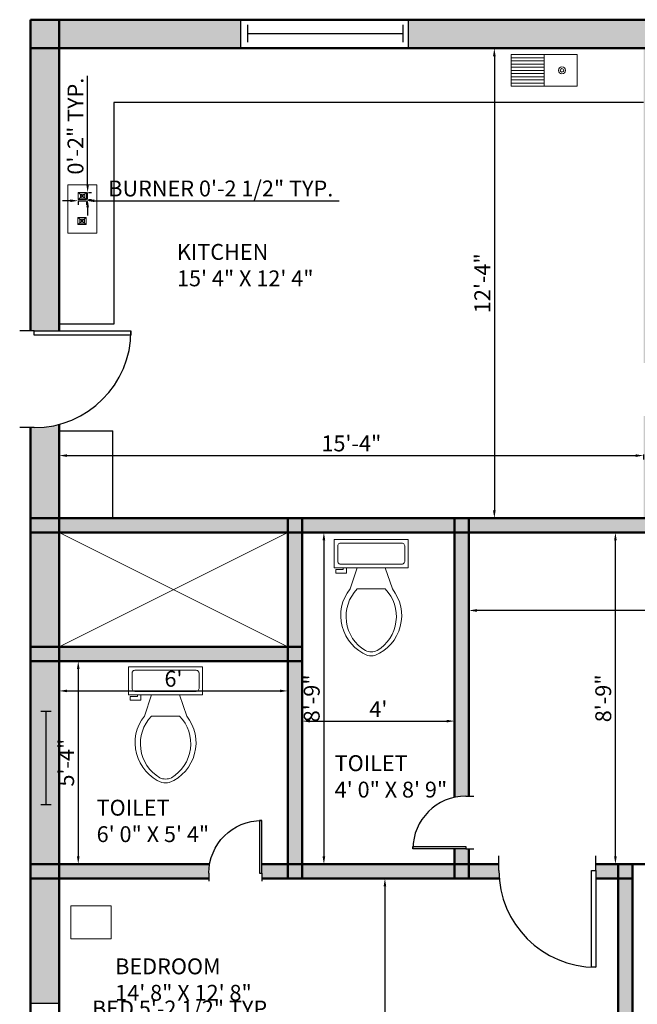
# Model space of a CAD drawing. Units: millimetres. Extents: x 3107 to 3757, y 777 to 1464.
# Tile 4 of 7: x 3107 to 3301, y 1140 to 1450. Entities that reach past the tile are written whole.
import ezdxf

# ---------------------------------------------------------------- set-up
doc = ezdxf.new("R2010")
doc.units = ezdxf.units.MM
for name, color, linetype, lineweight in [('A-ANNO-DIMS', 50, 'Continuous', 18), ('A-AREA-IDEN', 160, 'Continuous', 18), ('A-EQPM', 140, 'Continuous', 18), ('A-FLOR-CASE', 140, 'Continuous', 25), ('A-FLOR-FIXT', 140, 'Continuous', 18), ('A-FLOR-OPEN', 8, 'Continuous', 18), ('A-WALL-PATT', 80, 'Continuous', 13), ('doors', 10, 'Continuous', 25), ('furniture', 140, 'Continuous', 18), ('walls', 80, 'Continuous', 50), ('windows', 30, 'Continuous', 25)]:
    doc.layers.add(name, color=color, linetype=linetype, lineweight=lineweight)
doc.styles.get("Standard").update_dxf_attribs({"font": 'arial.ttf'})
doc.dimstyles.new('ISO-25', dxfattribs={"dimtxt": 5, "dimasz": 2.5, "dimexe": 1.25, "dimexo": 0.625, "dimtad": 1, "dimdec": 0, "dimlunit": 3, "dimtxsty": 'Standard', "dimcen": 2.5, "dimadec": 0, "dimazin": 0, "dimtfac": 1, "dimtdec": 0, "dimtmove": 0, "dimatfit": 3, "dimfxl": 1, "dimarcsym": 0})

# ---------------------------------------------------------------- blocks, each defined once
blk = doc.blocks.new('*U2')
for p, q in [((0, 0), (0, -6)), ((40, 0), (40, -6))]:
    blk.add_line(p, q)
blk.add_lwpolyline([(0, 0), (0, 40), (1.75, 40), (1.75, 0)], close=True)
blk.add_arc((0, 0), 40, 0, 90)
blk = doc.blocks.new('*U4')
for p, q in [((0, 4), (0, 0)), ((36, 4), (36, 0)), ((0, 2), (36, 2))]:
    blk.add_line(p, q)
blk = doc.blocks.new('*U5')
for p, q in [((0, 4), (0, 0)), ((36, 4), (36, 0)), ((0, 2), (36, 2))]:
    blk.add_line(p, q)
blk = doc.blocks.new('Toilet - top')
for p, q in [((9.5, -6), (9.5, -2)), ((-8, -8.5), (-8, -8)), ((-7, -8), (-7, -9.5)), ((-4, -8), (-6, -14)), ((4, -8), (6, -14)), ((-10, -8.5), (-8, -8.5)), ((-10, -9.5), (-10, -8.5)), ((-7, -9.5), (-10, -9.5)), ((4, -14), (-4, -14))]:
    blk.add_line(p, q)
blk.add_lwpolyline([(10.5, -8), (10.5, 0), (-10.5, 0), (-10.5, -8)], close=True)
for points in [[(-9.5, -2), (-9.5, -6)], [(8.5, -1), (-8.5, -1)], [(-8.5, -7), (8.5, -7)]]:
    blk.add_lwpolyline(points)
for centre, radius, start, end in [((-8.62, -1.88), 0.884, 81.8699, 188.1301), ((8.62, -1.88), 0.884, 351.8699, 98.1301), ((-8.62, -6.12), 0.884, 171.8699, 278.1301), ((8.62, -6.12), 0.884, 261.8699, 8.1301), ((3.52, -21.58), 12.17, 141.4691, 247.9714), ((4.2, -21.82), 11.33, 136.3677, 238.9468), ((-3.52, -21.58), 12.17, 292.0284, 38.5307), ((-4.2, -21.82), 11.33, 301.053, 43.6321), ((0, -27.88), 4, 245.7318, 294.2682), ((0, -29), 4, 254.8605, 285.1395)]:
    blk.add_arc(centre, radius, start, end)
blk = doc.blocks.new('*D16')
at = {"layer": 'A-ANNO-DIMS', "color": 0, "lineweight": -2, "transparency": 16777216}
for p, q in [((3257.1, 1441.43), (3257.73, 1441.43)), ((3256.48, 1438.93), (3256.48, 1295.93)), ((3257.1, 1293.43), (3257.73, 1293.43))]:
    blk.add_line(p, q, dxfattribs=at)
at = {"layer": 'A-ANNO-DIMS', "color": 0, "transparency": 16777216}
for points in [[(3256.06, 1438.93), (3256.9, 1438.93), (3256.48, 1441.43)], [(3256.06, 1295.93), (3256.9, 1295.93), (3256.48, 1293.43)]]:
    blk.add_solid(points, dxfattribs=at)
at = {"layer": 'Defpoints', "color": 0, "transparency": 16777216}
for p in [(3256.48, 1441.43), (3256.48, 1293.43), (3256.48, 1293.43)]:
    blk.add_point(p, dxfattribs=at)
at = {"layer": 'A-ANNO-DIMS', "color": 0, "transparency": 16777216, "insert": (3253.34, 1367.43), "char_height": 5, "attachment_point": 5, "rotation": 90}
blk.add_mtext('12\'-4"', dxfattribs=at)
blk = doc.blocks.new('*D17')
at = {"layer": 'A-ANNO-DIMS', "color": 0, "lineweight": -2, "transparency": 16777216}
for p, q in [((3119.47, 1311.37), (3119.47, 1314.39)), ((3121.97, 1313.14), (3300.97, 1313.14)), ((3303.47, 1313.51), (3303.47, 1311.89))]:
    blk.add_line(p, q, dxfattribs=at)
at = {"layer": 'A-ANNO-DIMS', "color": 0, "transparency": 16777216}
for points in [[(3121.97, 1313.56), (3121.97, 1312.72), (3119.47, 1313.14)], [(3300.97, 1313.56), (3300.97, 1312.72), (3303.47, 1313.14)]]:
    blk.add_solid(points, dxfattribs=at)
at = {"layer": 'Defpoints', "color": 0, "transparency": 16777216}
for p in [(3303.47, 1314.14), (3303.47, 1313.14), (3119.47, 1310.75)]:
    blk.add_point(p, dxfattribs=at)
at = {"layer": 'A-ANNO-DIMS', "color": 0, "transparency": 16777216, "insert": (3211.47, 1316.32), "char_height": 5, "attachment_point": 5}
blk.add_mtext('15\'-4"', dxfattribs=at)
blk = doc.blocks.new('*D24')
at = {"layer": 'A-ANNO-DIMS', "color": 0, "lineweight": -2, "transparency": 16777216}
for p, q in [((3248.47, 1264.98), (3248.47, 1265.6)), ((3464.47, 1264.98), (3464.47, 1265.6)), ((3461.97, 1264.35), (3250.97, 1264.35))]:
    blk.add_line(p, q, dxfattribs=at)
at = {"layer": 'A-ANNO-DIMS', "color": 0, "transparency": 16777216}
for points in [[(3250.97, 1264.77), (3250.97, 1263.94), (3248.47, 1264.35)], [(3461.97, 1264.77), (3461.97, 1263.94), (3464.47, 1264.35)]]:
    blk.add_solid(points, dxfattribs=at)
at = {"layer": 'Defpoints', "color": 0, "transparency": 16777216}
for p in [(3248.47, 1264.35), (3248.47, 1264.35), (3464.47, 1264.35)]:
    blk.add_point(p, dxfattribs=at)
at = {"layer": 'A-ANNO-DIMS', "color": 0, "transparency": 16777216, "insert": (3356.47, 1267.53), "char_height": 5, "attachment_point": 5}
blk.add_mtext("18'", dxfattribs=at)
blk = doc.blocks.new('*D25')
at = {"layer": 'A-ANNO-DIMS', "color": 0, "lineweight": -2, "transparency": 16777216}
for p, q in [((3294.84, 1288.93), (3293.35, 1288.93)), ((3294.6, 1186.93), (3294.6, 1286.43)), ((3294.84, 1184.43), (3293.35, 1184.43))]:
    blk.add_line(p, q, dxfattribs=at)
at = {"layer": 'A-ANNO-DIMS', "color": 0, "transparency": 16777216}
for points in [[(3294.18, 1286.43), (3295.01, 1286.43), (3294.6, 1288.93)], [(3294.18, 1186.93), (3295.01, 1186.93), (3294.6, 1184.43)]]:
    blk.add_solid(points, dxfattribs=at)
at = {"layer": 'Defpoints', "color": 0, "transparency": 16777216}
for p in [(3294.6, 1288.93), (3295.47, 1288.93), (3295.47, 1184.43)]:
    blk.add_point(p, dxfattribs=at)
at = {"layer": 'A-ANNO-DIMS', "color": 0, "transparency": 16777216, "insert": (3291.42, 1236.68), "char_height": 5, "attachment_point": 5, "rotation": 90}
blk.add_mtext('8\'-9"', dxfattribs=at)
blk = doc.blocks.new('*D26')
at = {"layer": 'A-ANNO-DIMS', "color": 0, "lineweight": -2, "transparency": 16777216}
for p, q in [((3195.97, 1225.71), (3195.97, 1230.76)), ((3198.47, 1229.51), (3241.47, 1229.51)), ((3243.97, 1225.71), (3243.97, 1230.76))]:
    blk.add_line(p, q, dxfattribs=at)
at = {"layer": 'A-ANNO-DIMS', "color": 0, "transparency": 16777216}
for points in [[(3198.47, 1229.92), (3198.47, 1229.09), (3195.97, 1229.51)], [(3241.47, 1229.92), (3241.47, 1229.09), (3243.97, 1229.51)]]:
    blk.add_solid(points, dxfattribs=at)
at = {"layer": 'Defpoints', "color": 0, "transparency": 16777216}
for p in [(3243.97, 1229.51), (3195.97, 1225.08), (3243.97, 1225.08)]:
    blk.add_point(p, dxfattribs=at)
at = {"layer": 'A-ANNO-DIMS', "color": 0, "transparency": 16777216, "insert": (3219.97, 1232.63), "char_height": 5, "attachment_point": 5}
blk.add_mtext("4'", dxfattribs=at)
blk = doc.blocks.new('*D27')
at = {"layer": 'A-ANNO-DIMS', "color": 0, "lineweight": -2, "transparency": 16777216}
for p, q in [((3200.33, 1288.93), (3204.07, 1288.93)), ((3202.82, 1286.43), (3202.82, 1186.93)), ((3200.33, 1184.43), (3204.07, 1184.43))]:
    blk.add_line(p, q, dxfattribs=at)
at = {"layer": 'A-ANNO-DIMS', "color": 0, "transparency": 16777216}
for points in [[(3202.4, 1286.43), (3203.24, 1286.43), (3202.82, 1288.93)], [(3202.4, 1186.93), (3203.24, 1186.93), (3202.82, 1184.43)]]:
    blk.add_solid(points, dxfattribs=at)
at = {"layer": 'Defpoints', "color": 0, "transparency": 16777216}
for p in [(3199.7, 1288.93), (3199.7, 1184.43), (3202.82, 1184.43)]:
    blk.add_point(p, dxfattribs=at)
at = {"layer": 'A-ANNO-DIMS', "color": 0, "transparency": 16777216, "insert": (3199.64, 1236.68), "char_height": 5, "attachment_point": 5, "rotation": 90}
blk.add_mtext('8\'-9"', dxfattribs=at)
blk = doc.blocks.new('*D28')
at = {"layer": 'A-ANNO-DIMS', "color": 0, "lineweight": -2, "transparency": 16777216}
for p, q in [((3119.47, 1241.1), (3119.47, 1237.77)), ((3191.47, 1241.1), (3191.47, 1237.77)), ((3121.97, 1239.02), (3188.97, 1239.02))]:
    blk.add_line(p, q, dxfattribs=at)
at = {"layer": 'A-ANNO-DIMS', "color": 0, "transparency": 16777216}
for points in [[(3121.97, 1239.44), (3121.97, 1238.61), (3119.47, 1239.02)], [(3188.97, 1239.44), (3188.97, 1238.61), (3191.47, 1239.02)]]:
    blk.add_solid(points, dxfattribs=at)
at = {"layer": 'Defpoints', "color": 0, "transparency": 16777216}
for p in [(3119.47, 1241.72), (3191.47, 1241.72), (3191.47, 1239.02)]:
    blk.add_point(p, dxfattribs=at)
at = {"layer": 'A-ANNO-DIMS', "color": 0, "transparency": 16777216, "insert": (3155.47, 1242.2), "char_height": 5, "attachment_point": 5}
blk.add_mtext("6'", dxfattribs=at)
blk = doc.blocks.new('*D29')
at = {"layer": 'A-ANNO-DIMS', "color": 0, "lineweight": -2, "transparency": 16777216}
for p, q in [((3123.55, 1248.43), (3126.75, 1248.43)), ((3125.5, 1245.93), (3125.5, 1186.93)), ((3123.55, 1184.43), (3126.75, 1184.43))]:
    blk.add_line(p, q, dxfattribs=at)
at = {"layer": 'A-ANNO-DIMS', "color": 0, "transparency": 16777216}
for points in [[(3125.08, 1245.93), (3125.91, 1245.93), (3125.5, 1248.43)], [(3125.08, 1186.93), (3125.91, 1186.93), (3125.5, 1184.43)]]:
    blk.add_solid(points, dxfattribs=at)
at = {"layer": 'Defpoints', "color": 0, "transparency": 16777216}
for p in [(3122.92, 1248.43), (3122.92, 1184.43), (3125.5, 1184.43)]:
    blk.add_point(p, dxfattribs=at)
at = {"layer": 'A-ANNO-DIMS', "color": 0, "transparency": 16777216, "insert": (3122.33, 1216.43), "char_height": 5, "attachment_point": 5, "rotation": 90}
blk.add_mtext('5\'-4"', dxfattribs=at)
blk = doc.blocks.new('*D33')
at = {"layer": 'A-ANNO-DIMS', "color": 0, "lineweight": -2, "transparency": 16777216}
for p, q in [((3221.28, 1179.93), (3223.29, 1179.93)), ((3222.04, 1177.43), (3222.04, 1030.43)), ((3221.28, 1027.93), (3223.29, 1027.93))]:
    blk.add_line(p, q, dxfattribs=at)
at = {"layer": 'A-ANNO-DIMS', "color": 0, "transparency": 16777216}
for points in [[(3221.62, 1177.43), (3222.45, 1177.43), (3222.04, 1179.93)], [(3221.62, 1030.43), (3222.45, 1030.43), (3222.04, 1027.93)]]:
    blk.add_solid(points, dxfattribs=at)
at = {"layer": 'Defpoints', "color": 0, "transparency": 16777216}
for p in [(3220.65, 1179.93), (3220.65, 1027.93), (3222.04, 1027.93)]:
    blk.add_point(p, dxfattribs=at)
at = {"layer": 'A-ANNO-DIMS', "color": 0, "transparency": 16777216, "insert": (3218.86, 1103.93), "char_height": 5, "attachment_point": 5, "rotation": 90}
blk.add_mtext('12\'-8"', dxfattribs=at)
blk = doc.blocks.new('COOKTOP-BURNER')
for p, q in [((0, 2.24), (2.56, 0)), ((2.56, 2.24), (0, 0))]:
    blk.add_line(p, q)
for points in [[(0, 2.24), (2.56, 2.24), (2.56, 0), (0, 0)], [(0.66, 1.7), (2.06, 1.7), (2.06, 0.46), (0.66, 0.46)]]:
    blk.add_lwpolyline(points, close=True)
blk = doc.blocks.new('*D49')
at = {"layer": 'A-ANNO-DIMS', "color": 0, "lineweight": -2, "transparency": 16777216}
for p, q in [((3127.01, 1126.35), (3127.01, 1136.38)), ((3187.19, 1135.13), (3129.51, 1135.13)), ((3189.69, 1126.35), (3189.69, 1136.38))]:
    blk.add_line(p, q, dxfattribs=at)
at = {"layer": 'A-ANNO-DIMS', "color": 0, "transparency": 16777216}
for points in [[(3129.51, 1135.55), (3129.51, 1134.71), (3127.01, 1135.13)], [(3187.19, 1135.55), (3187.19, 1134.71), (3189.69, 1135.13)]]:
    blk.add_solid(points, dxfattribs=at)
at = {"layer": 'Defpoints', "color": 0, "transparency": 16777216}
for p in [(3127.01, 1135.13), (3127.01, 1125.73), (3189.69, 1125.73)]:
    blk.add_point(p, dxfattribs=at)
at = {"layer": 'A-ANNO-DIMS', "color": 0, "transparency": 16777216, "insert": (3158.35, 1138.34), "char_height": 5, "attachment_point": 5}
blk.add_mtext('BED 5\'-2 1/2" TYP.', dxfattribs=at)
blk = doc.blocks.new('*D61')
at = {"layer": 'A-ANNO-DIMS', "color": 0, "lineweight": -2, "transparency": 16777216}
for p, q in [((3123, 1393.41), (3120.5, 1393.41)), ((3125.5, 1393.41), (3128.06, 1393.41)), ((3125.5, 1393.17), (3125.5, 1392.16)), ((3128.06, 1393.17), (3128.06, 1392.16)), ((3130.56, 1393.41), (3207.66, 1393.41))]:
    blk.add_line(p, q, dxfattribs=at)
at = {"layer": 'A-ANNO-DIMS', "color": 0, "transparency": 16777216}
for points in [[(3123, 1393.83), (3123, 1393), (3125.5, 1393.41)], [(3130.56, 1393.83), (3130.56, 1393), (3128.06, 1393.41)]]:
    blk.add_solid(points, dxfattribs=at)
at = {"layer": 'Defpoints', "color": 0, "transparency": 16777216}
for p in [(3125.5, 1393.8), (3128.06, 1393.8), (3128.06, 1393.41)]:
    blk.add_point(p, dxfattribs=at)
at = {"layer": 'A-ANNO-DIMS', "color": 0, "transparency": 16777216, "insert": (3170.36, 1396.62), "char_height": 5, "attachment_point": 5}
blk.add_mtext('BURNER 0\'-2 1/2" TYP.', dxfattribs=at)
blk = doc.blocks.new('*D62')
at = {"layer": 'A-ANNO-DIMS', "color": 0, "lineweight": -2, "transparency": 16777216}
for p, q in [((3128.45, 1398.53), (3128.45, 1432.76)), ((3128.45, 1393.8), (3128.45, 1396.03)), ((3128.69, 1396.03), (3129.7, 1396.03)), ((3128.69, 1393.8), (3129.7, 1393.8)), ((3128.45, 1391.3), (3128.45, 1388.8))]:
    blk.add_line(p, q, dxfattribs=at)
at = {"layer": 'A-ANNO-DIMS', "color": 0, "transparency": 16777216}
for points in [[(3128.03, 1398.53), (3128.87, 1398.53), (3128.45, 1396.03)], [(3128.03, 1391.3), (3128.87, 1391.3), (3128.45, 1393.8)]]:
    blk.add_solid(points, dxfattribs=at)
at = {"layer": 'Defpoints', "color": 0, "transparency": 16777216}
for p in [(3128.06, 1396.03), (3128.45, 1396.03), (3128.06, 1393.8)]:
    blk.add_point(p, dxfattribs=at)
at = {"layer": 'A-ANNO-DIMS', "color": 0, "transparency": 16777216, "insert": (3125.27, 1416.9), "char_height": 5, "attachment_point": 5, "rotation": 90}
blk.add_mtext('0\'-2" TYP.', dxfattribs=at)

msp = doc.modelspace()

# ---------------------------------------------------------------- hatches: boundary and pattern name
at = {"layer": 'A-WALL-PATT'}
h = msp.add_hatch(color=256, dxfattribs=at)
h.dxf.hatch_style = 1
h.paths.add_polyline_path([(3119.47, 1087.39), (3110.47, 1087.39), (3110.47, 1027.93), (3119.47, 1027.93)])
h.paths.add_polyline_path([(3119.47, 1027.93), (3110.47, 1027.93), (3110.47, 1023.43), (3119.47, 1023.43)])
h.paths.add_polyline_path([(3267.47, 1027.93), (3119.47, 1027.93), (3119.47, 1023.43), (3267.47, 1023.43)])
h.paths.add_polyline_path([(3119.47, 1023.43), (3110.47, 1023.43), (3110.47, 979.44), (3119.47, 979.44)])
h.paths.add_polyline_path([(3299.97, 1179.93), (3295.47, 1179.93), (3295.47, 1027.93), (3299.97, 1027.93)])
h.paths.add_polyline_path([(3295.47, 1027.93), (3271.97, 1027.93), (3271.97, 1023.43), (3295.47, 1023.43)])
h.paths.add_polyline_path([(3271.97, 1027.93), (3267.47, 1027.93), (3267.47, 1023.43), (3271.97, 1023.43)])
h.paths.add_polyline_path([(3299.97, 1027.93), (3295.47, 1027.93), (3295.47, 1023.43), (3299.97, 1023.43)])
h.paths.add_polyline_path([(3299.97, 1184.43), (3295.47, 1184.43), (3295.47, 1179.93), (3299.97, 1179.93)])
h.paths.add_polyline_path([(3295.47, 1184.43), (3288.38, 1184.43), (3288.38, 1182.47), (3288.38, 1179.93), (3295.47, 1179.93)])
h.paths.add_polyline_path([(3352.47, 1179.93), (3347.97, 1179.93), (3347.97, 1027.93), (3352.47, 1027.93)])
h.paths.add_polyline_path([(3352.47, 1184.43), (3347.97, 1184.43), (3347.97, 1179.93), (3352.47, 1179.93)])
h.paths.add_polyline_path([(3464.47, 1184.43), (3352.47, 1184.43), (3352.47, 1179.93), (3464.47, 1179.93)])
h.paths.add_polyline_path([(3468.97, 1288.93), (3464.47, 1288.93), (3464.47, 1184.43), (3468.97, 1184.43)])
h.paths.add_polyline_path([(3468.97, 1184.43), (3464.47, 1184.43), (3464.47, 1179.93), (3468.97, 1179.93)])
h.paths.add_polyline_path([(3195.97, 1248.43), (3191.47, 1248.43), (3191.47, 1184.43), (3195.97, 1184.43)])
h.paths.add_polyline_path([(3195.97, 1184.43), (3191.47, 1184.43), (3191.47, 1179.93), (3195.97, 1179.93)])
h.paths.add_polyline_path([(3191.47, 1184.43), (3183.28, 1184.43), (3183.28, 1181.58), (3183.28, 1179.93), (3191.47, 1179.93)])
h.paths.add_polyline_path([(3243.97, 1184.43), (3195.97, 1184.43), (3195.97, 1179.93), (3243.97, 1179.93)])
h.paths.add_polyline_path([(3257.91, 1182.47), (3257.91, 1184.43), (3248.47, 1184.43), (3248.47, 1179.93), (3258.02, 1179.93, -0.020891)])
h.paths.add_polyline_path([(3248.47, 1184.43), (3243.97, 1184.43), (3243.97, 1179.93), (3248.47, 1179.93)])
h.paths.add_polyline_path([(3248.47, 1189.24), (3247.51, 1189.24), (3243.97, 1189.24), (3243.97, 1184.43), (3248.47, 1184.43)])
h.paths.add_polyline_path([(3166.87, 1184.43), (3119.47, 1184.43), (3119.47, 1179.93), (3166.63, 1179.93), (3166.63, 1181.58, -0.042981)])
h.paths.add_polyline_path([(3119.47, 1184.43), (3110.47, 1184.43), (3110.47, 1179.93), (3119.47, 1179.93)])
h.paths.add_polyline_path([(3119.47, 1248.43), (3110.47, 1248.43), (3110.47, 1184.43), (3119.47, 1184.43)])
h.paths.add_polyline_path([(3119.47, 1179.93), (3110.47, 1179.93), (3110.47, 1140.65), (3119.47, 1140.65)])
h.paths.add_polyline_path([(3119.47, 1288.93), (3110.47, 1288.93), (3110.47, 1252.93), (3119.47, 1252.93)])
h.paths.add_polyline_path([(3119.47, 1252.93), (3110.47, 1252.93), (3110.47, 1248.43), (3119.47, 1248.43)])
h.paths.add_polyline_path([(3191.47, 1252.93), (3119.47, 1252.93), (3119.47, 1248.43), (3191.47, 1248.43)])
h.paths.add_polyline_path([(3195.97, 1288.93), (3191.47, 1288.93), (3191.47, 1252.93), (3195.97, 1252.93)])
h.paths.add_polyline_path([(3195.97, 1252.93), (3191.47, 1252.93), (3191.47, 1248.43), (3195.97, 1248.43)])
h.paths.add_polyline_path([(3248.47, 1293.43), (3243.97, 1293.43), (3243.97, 1288.93), (3248.47, 1288.93)])
h.paths.add_polyline_path([(3243.97, 1293.43), (3195.97, 1293.43), (3195.97, 1288.93), (3243.97, 1288.93)])
h.paths.add_polyline_path([(3303.47, 1293.43), (3248.47, 1293.43), (3248.47, 1288.93), (3303.47, 1288.93)])
h.paths.add_polyline_path([(3248.47, 1288.93), (3243.97, 1288.93), (3243.97, 1205.51, -0.053712), (3247.51, 1205.89), (3248.47, 1205.89)])
h.paths.add_polyline_path([(3191.47, 1293.43), (3119.47, 1293.43), (3119.47, 1288.93), (3191.47, 1288.93)])
h.paths.add_polyline_path([(3119.47, 1293.43), (3110.47, 1293.43), (3110.47, 1288.93), (3119.47, 1288.93)])
h.paths.add_polyline_path([(3119.47, 1322.96, -0.065064), (3111.64, 1321.93), (3110.47, 1321.93), (3110.47, 1293.43), (3119.47, 1293.43)])
h.paths.add_polyline_path([(3195.97, 1293.43), (3191.47, 1293.43), (3191.47, 1288.93), (3195.97, 1288.93)])
h.paths.add_polyline_path([(3119.47, 1450.43), (3110.47, 1450.43), (3110.47, 1441.43), (3119.47, 1441.43)])
h.paths.add_polyline_path([(3119.47, 1441.43), (3110.47, 1441.43), (3110.47, 1352.4), (3111.64, 1352.4), (3119.47, 1352.4)])
h.paths.add_polyline_path([(3176.58, 1450.43), (3119.47, 1450.43), (3119.47, 1441.43), (3176.58, 1441.43)])
h.paths.add_polyline_path([(3323.19, 1450.43), (3307.97, 1450.43), (3307.97, 1441.43), (3323.19, 1441.43)])
h.paths.add_polyline_path([(3307.97, 1450.43), (3303.47, 1450.43), (3303.47, 1441.43), (3307.97, 1441.43)])
h.paths.add_polyline_path([(3303.47, 1450.43), (3229.4, 1450.43), (3229.4, 1441.43), (3303.47, 1441.43)])
h.paths.add_polyline_path([(3307.97, 1441.43), (3303.47, 1441.43), (3303.47, 1363.43), (3307.97, 1363.43)])
h.paths.add_polyline_path([(3307.97, 1363.43), (3303.47, 1363.43), (3303.47, 1358.93), (3307.97, 1358.93)])
h.paths.add_polyline_path([(3307.97, 1358.93), (3303.47, 1358.93), (3303.47, 1342.3), (3305.5, 1342.3, -0.037178), (3307.97, 1342.12)])
h.paths.add_polyline_path([(3379.97, 1363.43), (3307.97, 1363.43), (3307.97, 1358.93), (3379.97, 1358.93)])
h.paths.add_polyline_path([(3384.47, 1393.61), (3383.04, 1393.61), (3379.97, 1393.61), (3379.97, 1363.43), (3384.47, 1363.43)])
h.paths.add_polyline_path([(3384.47, 1363.43), (3379.97, 1363.43), (3379.97, 1358.93), (3384.47, 1358.93)])
h.paths.add_polyline_path([(3384.47, 1358.93), (3379.97, 1358.93), (3379.97, 1293.43), (3384.47, 1293.43)])
h.paths.add_polyline_path([(3384.47, 1441.43), (3379.97, 1441.43), (3379.97, 1409.98, -0.046389), (3383.04, 1410.27), (3384.47, 1410.27)])
h.paths.add_polyline_path([(3384.47, 1450.43), (3379.97, 1450.43), (3379.97, 1441.43), (3384.47, 1441.43)])
h.paths.add_polyline_path([(3379.97, 1450.43), (3357.18, 1450.43), (3357.18, 1441.43), (3379.97, 1441.43)])
h.paths.add_polyline_path([(3432.79, 1450.43), (3384.47, 1450.43), (3384.47, 1441.43), (3432.79, 1441.43)])
h.paths.add_polyline_path([(3540.47, 1450.43), (3484.18, 1450.43), (3484.18, 1441.43), (3540.47, 1441.43)])
h.paths.add_polyline_path([(3544.97, 1450.43), (3540.47, 1450.43), (3540.47, 1441.43), (3544.97, 1441.43)])
h.paths.add_polyline_path([(3544.97, 1441.43), (3540.47, 1441.43), (3540.47, 1293.43), (3544.97, 1293.43)])
h.paths.add_polyline_path([(3590.83, 1450.43), (3544.97, 1450.43), (3544.97, 1441.43), (3590.83, 1441.43)])
h.paths.add_polyline_path([(3712.97, 1450.43), (3645.62, 1450.43), (3645.62, 1441.43), (3712.97, 1441.43)])
h.paths.add_polyline_path([(3721.97, 1441.43), (3712.97, 1441.43), (3712.97, 1288.93), (3712.97, 1184.43), (3721.97, 1184.43), (3721.97, 1288.93)])
h.paths.add_polyline_path([(3721.97, 1450.43), (3712.97, 1450.43), (3712.97, 1441.43), (3721.97, 1441.43)])
h.paths.add_polyline_path([(3712.97, 1184.43), (3658.24, 1184.43), (3658.24, 1183.15), (3658.24, 1179.93), (3712.97, 1179.93)])
h.paths.add_polyline_path([(3721.97, 1184.43), (3712.97, 1184.43), (3712.97, 1179.93), (3721.97, 1179.93)])
h.paths.add_polyline_path([(3597.32, 1183.15), (3597.32, 1184.43), (3544.97, 1184.43), (3544.97, 1179.93), (3597.32, 1179.93)])
h.paths.add_polyline_path([(3544.97, 1184.43), (3540.47, 1184.43), (3540.47, 1179.93), (3544.97, 1179.93)])
h.paths.add_polyline_path([(3544.97, 1179.93), (3540.47, 1179.93), (3540.47, 1143.69), (3543.65, 1143.69), (3544.97, 1143.69)])
h.paths.add_polyline_path([(3721.97, 1179.93), (3712.97, 1179.93), (3712.97, 1006.22), (3712.97, 871.43), (3721.97, 871.43), (3721.97, 1006.22)])
h.paths.add_polyline_path([(3468.97, 1293.43), (3464.47, 1293.43), (3464.47, 1288.93), (3468.97, 1288.93)])
h.paths.add_polyline_path([(3540.47, 1293.43), (3468.97, 1293.43), (3468.97, 1288.93), (3540.47, 1288.93)])
h.paths.add_polyline_path([(3544.97, 1293.43), (3540.47, 1293.43), (3540.47, 1288.93), (3544.97, 1288.93)])
h.paths.add_polyline_path([(3464.47, 1293.43), (3417.83, 1293.43, -0.015057), (3417.88, 1291.6), (3417.88, 1288.93), (3464.47, 1288.93)])
h.paths.add_polyline_path([(3379.97, 1293.43), (3307.97, 1293.43), (3307.97, 1288.93), (3379.97, 1288.93)])
h.paths.add_polyline_path([(3307.97, 1325.65), (3305.5, 1325.65), (3303.47, 1325.65), (3303.47, 1293.43), (3307.97, 1293.43)])
h.paths.add_polyline_path([(3307.97, 1293.43), (3303.47, 1293.43), (3303.47, 1288.93), (3307.97, 1288.93)])
h.paths.add_polyline_path([(3384.47, 1293.43), (3379.97, 1293.43), (3379.97, 1288.93), (3384.47, 1288.93)])
h.paths.add_polyline_path([(3387.42, 1291.6), (3387.42, 1293.43), (3384.47, 1293.43), (3384.47, 1288.93), (3387.42, 1288.93)])
h.paths.add_polyline_path([(3119.47, 927.28), (3110.47, 927.28), (3110.47, 871.43), (3119.47, 871.43)])
h.paths.add_polyline_path([(3119.47, 871.43), (3110.47, 871.43), (3110.47, 862.43), (3119.47, 862.43)])
h.paths.add_polyline_path([(3267.47, 871.43), (3119.47, 871.43), (3119.47, 862.43), (3267.47, 862.43)])
h.paths.add_polyline_path([(3271.97, 971.43), (3267.47, 971.43), (3267.47, 871.43), (3271.97, 871.43)])
h.paths.add_polyline_path([(3271.97, 871.43), (3267.47, 871.43), (3267.47, 862.43), (3271.97, 862.43)])
h.paths.add_polyline_path([(3287.13, 871.43), (3271.97, 871.43), (3271.97, 862.43), (3287.13, 862.43)])
h.paths.add_polyline_path([(3347.97, 871.43), (3318.96, 871.43), (3318.96, 862.43), (3347.97, 862.43)])
h.paths.add_polyline_path([(3352.47, 971.43), (3347.97, 971.43), (3347.97, 871.43), (3352.47, 871.43)])
h.paths.add_polyline_path([(3352.47, 871.43), (3347.97, 871.43), (3347.97, 862.43), (3352.47, 862.43)])
h.paths.add_polyline_path([(3375.96, 871.43), (3352.47, 871.43), (3352.47, 862.43), (3375.96, 862.43)])
h.paths.add_polyline_path([(3352.47, 975.93), (3347.97, 975.93), (3347.97, 971.43), (3352.47, 971.43)])
h.paths.add_polyline_path([(3352.47, 986.27, -0.01722), (3350.37, 986.2), (3347.97, 986.2), (3347.97, 975.93), (3352.47, 975.93)])
h.paths.add_polyline_path([(3347.97, 975.93), (3292.38, 975.93), (3292.38, 973.47, -0.030785), (3292.25, 971.43), (3347.97, 971.43)])
h.paths.add_polyline_path([(3271.97, 985.98), (3269.95, 985.98), (3267.47, 985.98), (3267.47, 975.93), (3271.97, 975.93)])
h.paths.add_polyline_path([(3271.97, 975.93), (3267.47, 975.93), (3267.47, 971.43), (3271.97, 971.43)])
h.paths.add_polyline_path([(3275.72, 975.93), (3271.97, 975.93), (3271.97, 971.43), (3275.72, 971.43), (3275.72, 973.47)])
h.paths.add_polyline_path([(3271.97, 1023.43), (3267.47, 1023.43), (3267.47, 1016.34, -0.020418), (3269.95, 1016.44), (3271.97, 1016.44)])
h.paths.add_polyline_path([(3352.47, 1023.43), (3347.97, 1023.43), (3347.97, 1016.67), (3350.37, 1016.67), (3352.47, 1016.67)])
h.paths.add_polyline_path([(3352.47, 1027.93), (3347.97, 1027.93), (3347.97, 1023.43), (3352.47, 1023.43)])
h.paths.add_polyline_path([(3476.47, 1027.93), (3352.47, 1027.93), (3352.47, 1023.43), (3476.47, 1023.43)])
h.paths.add_polyline_path([(3540.47, 1027.93), (3480.97, 1027.93), (3480.97, 1023.43), (3540.47, 1023.43)])
h.paths.add_polyline_path([(3480.97, 1027.93), (3476.47, 1027.93), (3476.47, 1023.43), (3480.97, 1023.43)])
h.paths.add_polyline_path([(3480.97, 1023.43), (3476.47, 1023.43), (3476.47, 871.43), (3480.97, 871.43)])
h.paths.add_polyline_path([(3476.47, 871.43), (3429.88, 871.43), (3429.88, 862.43), (3476.47, 862.43)])
h.paths.add_polyline_path([(3480.97, 871.43), (3476.47, 871.43), (3476.47, 862.43), (3480.97, 862.43)])
h.paths.add_polyline_path([(3493.81, 871.43), (3480.97, 871.43), (3480.97, 862.43), (3493.81, 862.43)])
h.paths.add_polyline_path([(3712.97, 871.43), (3525.61, 871.43), (3525.61, 862.43), (3712.97, 862.43)])
h.paths.add_polyline_path([(3721.97, 871.43), (3712.97, 871.43), (3712.97, 862.43), (3721.97, 862.43)])

# ---------------------------------------------------------------- linework, layer by layer
at = {"layer": 'A-EQPM'}
msp.add_lwpolyline([(3122.19, 1398.44), (3131.33, 1398.44), (3131.33, 1383.16), (3122.19, 1383.16)], close=True, dxfattribs=at)
at = {"layer": 'A-FLOR-CASE'}
for p, q in [((3303.47, 1424.33), (3136.75, 1424.33)), ((3136.75, 1424.33), (3136.75, 1354.51)), ((3136.75, 1354.51), (3119.47, 1354.51)), ((3119.47, 1320.97), (3136.43, 1320.97)), ((3136.43, 1293.43), (3136.43, 1320.97)), ((3119.47, 1293.43), (3136.43, 1293.43))]:
    msp.add_line(p, q, dxfattribs=at)
at = {"layer": 'A-FLOR-FIXT'}
for p, q in [((3261.77, 1439.45), (3272.15, 1439.45)), ((3272.15, 1439.45), (3272.15, 1429.49)), ((3261.77, 1438.45), (3272.15, 1438.45)), ((3261.77, 1437.45), (3272.15, 1437.45)), ((3261.77, 1436.45), (3272.15, 1436.45)), ((3261.77, 1435.45), (3272.15, 1435.45)), ((3261.77, 1434.45), (3272.15, 1434.45)), ((3261.77, 1433.45), (3272.15, 1433.45)), ((3261.77, 1432.45), (3272.15, 1432.45)), ((3261.77, 1431.45), (3272.15, 1431.45)), ((3261.77, 1430.45), (3272.15, 1430.45))]:
    msp.add_line(p, q, dxfattribs=at)
msp.add_lwpolyline([(3261.77, 1439.45), (3282.53, 1439.45), (3282.53, 1429.49), (3261.77, 1429.49)], close=True, dxfattribs=at)
for radius in [1.11, 0.558]:
    msp.add_circle((3277.77, 1434.47), radius, dxfattribs=at)
at = {"layer": 'A-FLOR-OPEN'}
for p, q in [((3119.47, 1288.93), (3191.47, 1252.93)), ((3191.47, 1288.93), (3119.47, 1252.93))]:
    msp.add_line(p, q, dxfattribs=at)
at = {"layer": 'furniture'}
msp.add_lwpolyline([(3123.17, 1171.31), (3135.83, 1171.31), (3135.83, 1160.91), (3123.17, 1160.91)], close=True, dxfattribs=at)
at = {"layer": 'walls'}
for p, q in [((3110.47, 1450.43), (3110.47, 1352.4)), ((3110.47, 1450.43), (3721.97, 1450.43)), ((3119.47, 1450.43), (3119.47, 1352.4)), ((3110.47, 1441.43), (3721.97, 1441.43)), ((3110.47, 1321.93), (3110.47, 862.43)), ((3119.47, 1322.96), (3119.47, 862.43)), ((3110.47, 1293.43), (3384.47, 1293.43)), ((3110.47, 1293.43), (3387.42, 1293.43)), ((3191.47, 1293.43), (3191.47, 1179.93)), ((3195.97, 1293.43), (3195.97, 1179.93)), ((3243.97, 1293.43), (3243.97, 1205.51)), ((3248.47, 1293.43), (3248.47, 1205.89)), ((3110.47, 1288.93), (3384.47, 1288.93)), ((3110.47, 1288.93), (3387.42, 1288.93)), ((3110.47, 1252.93), (3195.97, 1252.93)), ((3110.47, 1248.43), (3195.97, 1248.43)), ((3243.97, 1189.24), (3243.97, 1179.93)), ((3248.47, 1189.24), (3248.47, 1179.93)), ((3110.47, 1184.43), (3166.87, 1184.43)), ((3183.28, 1184.43), (3257.91, 1184.43)), ((3288.38, 1184.43), (3468.97, 1184.43)), ((3295.47, 1184.43), (3295.47, 1023.43)), ((3299.97, 1184.43), (3299.97, 1023.43)), ((3110.47, 1179.93), (3166.63, 1179.93)), ((3183.28, 1179.93), (3258.02, 1179.93)), ((3288.38, 1179.93), (3299.97, 1179.93))]:
    msp.add_line(p, q, dxfattribs=at)
at = {"layer": 'windows'}
for p, q in [((3176.58, 1450.43), (3176.58, 1441.43)), ((3229.4, 1450.43), (3229.4, 1441.43)), ((3110.47, 1140.65), (3119.47, 1140.65))]:
    msp.add_line(p, q, dxfattribs=at)

# ---------------------------------------------------------------- block references
at = {"layer": 'A-EQPM'}
for p in [(3125.5, 1393.8), (3125.38, 1385.88)]:
    msp.add_blockref('COOKTOP-BURNER', p, dxfattribs=at)
at = {"layer": 'A-FLOR-FIXT', "xscale": 1.109949414103811, "yscale": 1.109949414103811, "zscale": 1.109949414103811}
for p in [(3217.72, 1286.69), (3152.98, 1246.65)]:
    msp.add_blockref('Toilet - top', p, dxfattribs=at)
at = {"layer": 'doors'}
for p, xscale, yscale, zscale, rotation in [((3111.64, 1352.4), 0.7615706373352984, 0.7615706373352984, 0.7615706373352984, 270), ((3247.51, 1189.24), 0.4163085604342208, 0.4163085604342208, 0.4163085604342208, 90.00000000000003), ((3288.38, 1182.47), 0.7615706373352984, 0.7615706373352984, 0.7615706373352984, 180)]:
    msp.add_blockref('*U2', p, dxfattribs=dict(at, xscale=xscale, yscale=yscale, zscale=zscale, rotation=rotation))
at = {"layer": 'doors', "xscale": -0.4163085604342208, "yscale": 0.4163085604342208, "zscale": 0.4163085604342208}
msp.add_blockref('*U2', (3183.28, 1181.58), dxfattribs=at)
at = {"layer": 'windows', "xscale": 1.357941570966636, "yscale": 1.357941570966636, "zscale": 1.357941570966636}
msp.add_blockref('*U4', (3178.82, 1443.34), dxfattribs=at)
at = {"layer": 'windows', "xscale": 0.8150463067894532, "yscale": 0.8150463067894532, "zscale": 0.8150463067894532, "rotation": 90}
msp.add_blockref('*U5', (3117, 1203.29), dxfattribs=at)

# ---------------------------------------------------------------- texts
at = {"layer": 'A-AREA-IDEN', "char_height": 5, "attachment_point": 1}
for s, width, insert in [('KITCHEN\\P15\' 4" X 12\' 4"', 68.2161, (3156.57, 1379.79)), ('TOILET\\P4\' 0" X 8\' 9"', 37.7453, (3206.22, 1218.77)), ('TOILET \\P6\' 0" X 5\' 4"', 40.2219, (3131.28, 1204.74)), ('BEDROOM\\P14\' 8" X 12\' 8"', 53.4954, (3137.13, 1154.77))]:
    msp.add_mtext_dynamic_manual_height_columns(s, width=width, gutter_width=12.5, heights=[0], dxfattribs=dict(at, insert=insert))

# ---------------------------------------------------------------- dimensions: what is measured, and where the dimension line sits
at = {"layer": 'A-ANNO-DIMS'}
for base, p1, p2, picture, middle in [((3256.48, 1293.43), (3256.48, 1441.43), (3256.48, 1293.43), '*D16', (3253.34, 1367.43)), ((3202.82084342, 1184.42857409), (3199.7005936, 1288.92857409), (3199.7005936, 1184.42857409), '*D27', (3199.64297848, 1236.67857409)), ((3294.59748357, 1288.92857409), (3295.46513133, 1184.42857409), (3295.46513133, 1288.92857409), '*D25', (3291.41961863, 1236.67857409)), ((3125.5, 1184.43), (3122.92, 1248.43), (3122.92, 1184.43), '*D29', (3122.33, 1216.43)), ((3222.04, 1027.93), (3220.65, 1179.93), (3220.65, 1027.93), '*D33', (3218.86, 1103.93))]:
    dim = msp.add_linear_dim(base=base, p1=p1, p2=p2, angle=90, dimstyle='ISO-25', override={"dimclrd": 0, "dimclre": 0, "dimclrt": 0}, dxfattribs=at)
    dim.commit()
    dim.dimension.update_dxf_attribs({"geometry": picture, "text_midpoint": middle})
for base, p1, p2, angle, text, picture, middle in [((3128.45, 1396.03), (3128.06, 1393.8), (3128.06, 1396.03), 90, '<> TYP.', '*D62', (3125.27, 1416.9)), ((3127.01, 1135.13), (3189.69, 1125.73), (3127.01, 1125.73), 180, 'BED <> TYP.', '*D49', (3158.35, 1138.34))]:
    dim = msp.add_linear_dim(base=base, p1=p1, p2=p2, angle=angle, text=text, dimstyle='ISO-25', override={"dimdec": 1, "dimlfac": 1, "dimrnd": 0, "dimzin": 1, "dimdsep": 46, "dimlunit": 4, "dimfrac": 2}, dxfattribs=at)
    dim.commit()
    dim.dimension.update_dxf_attribs({"geometry": picture, "text_midpoint": middle})
dim = msp.add_linear_dim(base=(3128.06, 1393.41), p1=(3125.5, 1393.8), p2=(3128.06, 1393.8), text='BURNER <> TYP.', dimstyle='ISO-25', override={"dimdec": 1, "dimlfac": 1, "dimrnd": 0, "dimzin": 1, "dimdsep": 46, "dimlunit": 4, "dimfrac": 2}, dxfattribs=at)
dim.commit()
dim.dimension.update_dxf_attribs({"geometry": '*D61', "text_midpoint": (3170.36, 1396.62)})
for base, p1, p2, picture, middle in [((3303.47, 1313.14), (3119.47, 1310.75), (3303.47, 1314.14), '*D17', (3211.47, 1316.32)), ((3248.47, 1264.35), (3464.47, 1264.35), (3248.47, 1264.35), '*D24', (3356.47, 1267.53)), ((3191.47, 1239.02), (3119.47, 1241.72), (3191.47, 1241.72), '*D28', (3155.47, 1242.2)), ((3243.97, 1229.51), (3195.97, 1225.08), (3243.97, 1225.08), '*D26', (3219.97, 1232.63))]:
    dim = msp.add_linear_dim(base=base, p1=p1, p2=p2, dimstyle='ISO-25', override={"dimclrd": 0, "dimclre": 0, "dimclrt": 0}, dxfattribs=at)
    dim.commit()
    dim.dimension.update_dxf_attribs({"geometry": picture, "text_midpoint": middle})

doc.saveas('drawing.dxf')
